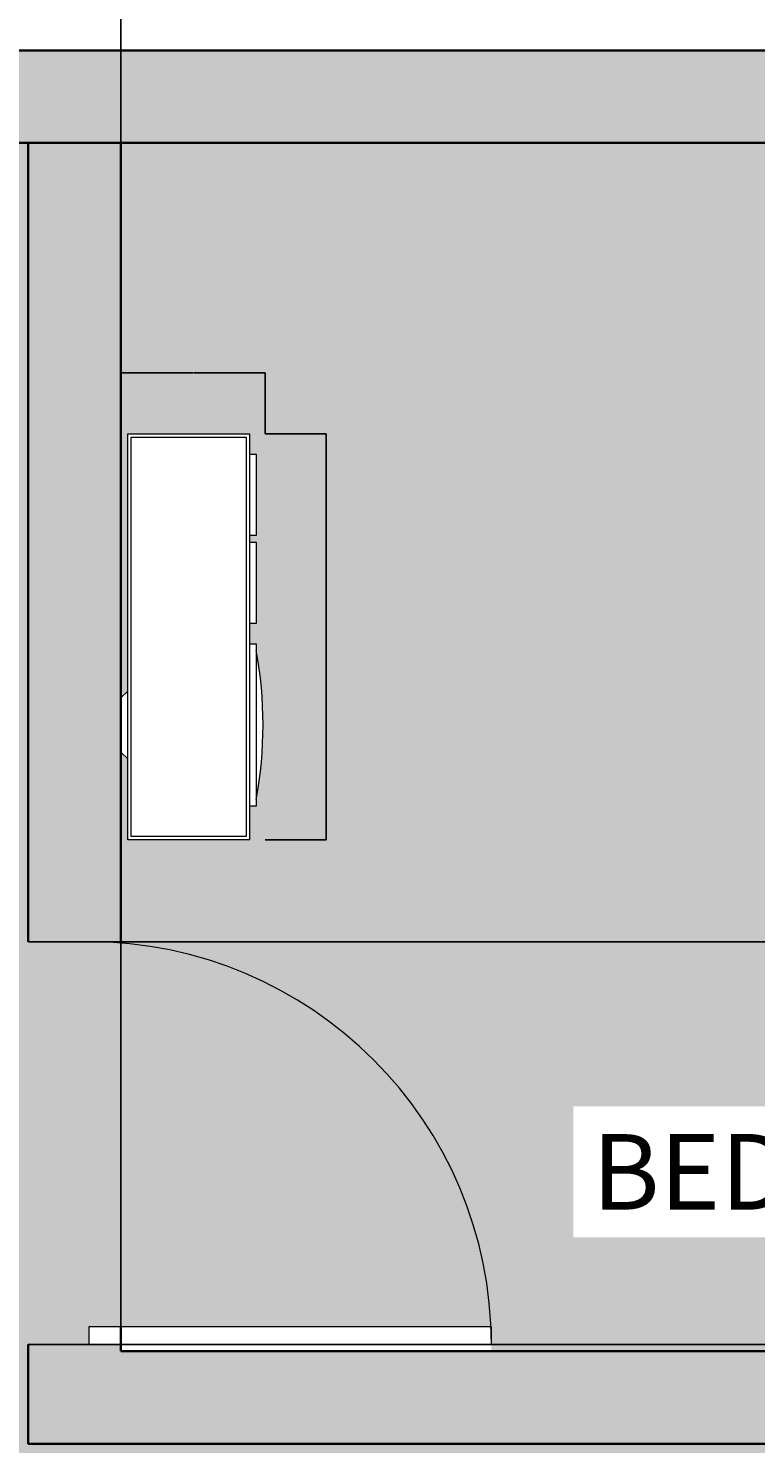
# Model space of a CAD drawing. Units: millimetres. Extents: x -229 to 16545, y -10488 to 4272.
# Tile 26 of 29: x 9556 to 11362, y -1208 to 2307. Entities that reach past the tile are written whole.
import ezdxf

# ---------------------------------------------------------------- set-up
doc = ezdxf.new("R2010")
doc.units = ezdxf.units.MM
for name, color, linetype, lineweight in [('A-ANNO-DIMS', 2, 'Continuous', 18), ('A-AREA-IDEN', 7, 'Continuous', 18), ('A-DOOR', 4, 'Continuous', 18), ('A-FURN', 8, 'Continuous', 18), ('A-WALL', 7, 'Continuous', 35)]:
    doc.layers.add(name, color=color, linetype=linetype, lineweight=lineweight)
doc.layers.add('A-FLOR-PATT', color=254, linetype='Continuous', lineweight=13, true_color=0xfeeab9)
doc.layers.add('A-WALL-PATT', color=18, linetype='Continuous', lineweight=13, true_color=0x000000)
doc.styles.get("Standard").update_dxf_attribs({"font": 'arial.ttf'})
doc.dimstyles.get("Standard").update_dxf_attribs({"dimtxt": 0.18, "dimasz": 0.18, "dimexe": 0.18, "dimexo": 0.0625, "dimgap": 0.09, "dimtad": 0, "dimtih": 1, "dimtoh": 1, "dimdec": 4, "dimzin": 0, "dimdsep": 46, "dimtxsty": 'Standard', "dimcen": 0.09, "dimadec": 0, "dimazin": 0, "dimtfac": 1, "dimtdec": 4, "dimtofl": 0, "dimtmove": 0, "dimatfit": 3, "dimfxl": 1, "dimtolj": 1, "dimtzin": 0, "dimarcsym": 0})

# ---------------------------------------------------------------- blocks, each defined once
blk = doc.blocks.new('Entertainment Center')
for p, q in [((-4, 0), (-5, -1)), ((4, 0), (-4, 0)), ((5, -1), (4, 0)), ((-17, -19), (-17, -1)), ((-17, -1), (43, -1)), ((-16.5, -18.5), (-16.5, -1.5)), ((-16.5, -1.5), (42.5, -1.5)), ((42.5, -1.5), (42.5, -18.5)), ((43, -1), (43, -19)), ((42.5, -18.5), (-16.5, -18.5)), ((43, -19), (-17, -19)), ((-12, -20), (-12, -19)), ((12, -20), (-12, -20)), ((12, -19), (12, -20)), ((15, -20), (15, -19)), ((27, -20), (15, -20)), ((27, -19), (27, -20)), ((28, -20), (28, -19)), ((40, -20), (28, -20)), ((40, -19), (40, -20))]:
    blk.add_line(p, q)
blk.add_arc((0, 40), 61, 259.6111, 280.3889)
blk = doc.blocks.new('*U13')
at = {"transparency": 33554687}
for p, q in [((0, 0), (0, -6)), ((-40, 0), (-40, -6))]:
    blk.add_line(p, q, dxfattribs=at)
blk.add_lwpolyline([(0, 0), (0, 40), (-1.75, 40), (-1.75, 0)], close=True, dxfattribs=at)
blk.add_arc((0, 0), 40, 90, 180, dxfattribs=at)
blk = doc.blocks.new('*D29')
at = {"layer": 'A-ANNO-DIMS', "color": 0, "lineweight": -2, "transparency": 16777216}
for p, q in [((10144.5, 1299.3), (10295.9, 1299.3)), ((10295.8, 1299.1), (10295.8, 795.3)), ((10295.8, 291.1), (10295.8, 794.9)), ((10144.5, 290.9), (10295.9, 290.9))]:
    blk.add_line(p, q, dxfattribs=at)
at = {"layer": 'A-ANNO-DIMS', "color": 0, "transparency": 16777216}
for points in [[(10295.7, 1299.1), (10295.8, 1299.1), (10295.8, 1299.3)], [(10295.7, 291.1), (10295.8, 291.1), (10295.8, 290.9)]]:
    blk.add_solid(points, dxfattribs=at)
at = {"layer": 'Defpoints', "color": 0, "transparency": 16777216}
for p in [(10144.5, 1299.3), (10295.8, 1299.3), (10144.5, 290.9)]:
    blk.add_point(p, dxfattribs=at)
at = {"layer": 'A-ANNO-DIMS', "color": 0, "transparency": 16777216, "insert": (10295.8, 795.1), "char_height": 0.18, "attachment_point": 5}
blk.add_mtext('\\A1;MEDIA UNIT 1008 TYP.', dxfattribs=at)
blk = doc.blocks.new('*D30')
at = {"layer": 'A-ANNO-DIMS', "color": 0, "lineweight": -2, "transparency": 16777216}
for p, q in [((9785.9, 1299.4), (9785.9, 1450.8)), ((9786.1, 1450.6), (9964.6, 1450.6)), ((10144.3, 1450.6), (9965.8, 1450.6)), ((10144.5, 1299.4), (10144.5, 1450.8))]:
    blk.add_line(p, q, dxfattribs=at)
at = {"layer": 'A-ANNO-DIMS', "color": 0, "transparency": 16777216}
for points in [[(9786.1, 1450.6), (9786.1, 1450.6), (9785.9, 1450.6)], [(10144.3, 1450.6), (10144.3, 1450.6), (10144.5, 1450.6)]]:
    blk.add_solid(points, dxfattribs=at)
at = {"layer": 'Defpoints', "color": 0, "transparency": 16777216}
for p in [(9785.9, 1450.6), (9785.9, 1299.3), (10144.5, 1299.3)]:
    blk.add_point(p, dxfattribs=at)
at = {"layer": 'A-ANNO-DIMS', "color": 0, "transparency": 16777216, "insert": (9965.2, 1450.6), "char_height": 0.18, "attachment_point": 5}
blk.add_mtext('\\A1;359 TYP.', dxfattribs=at)
blk = doc.blocks.new('*D45')
at = {"layer": 'A-ANNO-DIMS', "color": 0, "lineweight": -2, "transparency": 16777216}
for p, q in [((2015.9, 2251.8), (2015.9, 4271.7)), ((2016.1, 4271.5), (8015.5, 4271.5)), ((14015.8, 4271.5), (8016.4, 4271.5)), ((14015.9, 2251.8), (14015.9, 4271.7))]:
    blk.add_line(p, q, dxfattribs=at)
at = {"layer": 'A-ANNO-DIMS', "color": 0, "transparency": 16777216}
for points in [[(2016.1, 4271.5), (2016.1, 4271.4), (2015.9, 4271.5)], [(14015.8, 4271.5), (14015.8, 4271.4), (14015.9, 4271.5)]]:
    blk.add_solid(points, dxfattribs=at)
at = {"layer": 'Defpoints', "color": 0, "transparency": 16777216}
for p in [(14015.9, 4271.5), (2015.9, 2251.7), (14015.9, 2251.7)]:
    blk.add_point(p, dxfattribs=at)
at = {"layer": 'A-ANNO-DIMS', "color": 0, "transparency": 16777216, "insert": (8015.9, 4271.5), "char_height": 0.18, "attachment_point": 5}
blk.add_mtext('\\A1;12000', dxfattribs=at)
blk = doc.blocks.new('*D52')
at = {"layer": 'A-ANNO-DIMS', "color": 0, "lineweight": -2, "transparency": 16777216}
for p, q in [((9785.9, -978.2), (9785.9, 4271.7)), ((9786.1, 4271.5), (11785.6, 4271.5)), ((13785.8, 4271.5), (11786.3, 4271.5)), ((13785.9, -978.2), (13785.9, 4271.7))]:
    blk.add_line(p, q, dxfattribs=at)
at = {"layer": 'A-ANNO-DIMS', "color": 0, "transparency": 16777216}
for points in [[(9786.1, 4271.5), (9786.1, 4271.4), (9785.9, 4271.5)], [(13785.8, 4271.5), (13785.8, 4271.4), (13785.9, 4271.5)]]:
    blk.add_solid(points, dxfattribs=at)
at = {"layer": 'Defpoints', "color": 0, "transparency": 16777216}
for p in [(13785.9, 4271.5), (9785.9, -978.3), (13785.9, -978.3)]:
    blk.add_point(p, dxfattribs=at)
at = {"layer": 'A-ANNO-DIMS', "color": 0, "transparency": 16777216, "insert": (11785.9, 4271.5), "char_height": 0.18, "attachment_point": 5}
blk.add_mtext('\\A1;4000', dxfattribs=at)
blk = doc.blocks.new('*D66')
at = {"layer": 'A-ANNO-DIMS', "color": 0, "lineweight": -2, "transparency": 16777216}
for p, q in [((9556, 38.2), (16544.5, 38.2)), ((16544.3, 38), (16544.3, -461.6)), ((16544.3, -961.6), (16544.3, -462)), ((9556, -961.8), (16544.5, -961.8))]:
    blk.add_line(p, q, dxfattribs=at)
at = {"layer": 'A-ANNO-DIMS', "color": 0, "transparency": 16777216}
for points in [[(16544.3, 38), (16544.4, 38), (16544.3, 38.2)], [(16544.3, -961.6), (16544.4, -961.6), (16544.3, -961.8)]]:
    blk.add_solid(points, dxfattribs=at)
at = {"layer": 'Defpoints', "color": 0, "transparency": 16777216}
for p in [(9555.9, 38.2), (9555.9, -961.8), (16544.3, -961.8)]:
    blk.add_point(p, dxfattribs=at)
at = {"layer": 'A-ANNO-DIMS', "color": 0, "transparency": 16777216, "insert": (16544.3, -461.8), "char_height": 0.18, "attachment_point": 5}
blk.add_mtext('\\A1;1000', dxfattribs=at)

msp = doc.modelspace()

# ---------------------------------------------------------------- hatches: boundary and pattern name
at = {"layer": 'A-FLOR-PATT', "transparency": 33554592}
h = msp.add_hatch(color=256, dxfattribs=at)
h.dxf.hatch_style = 1
h.paths.add_polyline_path([(7975.933, -5325.772), (7943.121, -5325.772), (7943.121, -4576.49, 0.40145271), (7225.933, -5325.772, 0.40145271), (6508.746, -4576.49), (6508.746, -5325.772), (6475.933, -5325.772), (6475.933, -5438.272), (5975.933, -5438.272), (5975.933, -7267.724), (5975.933, -7438.272), (6478.619, -7438.272), (6463.448, -7355.919), (6464.88, -7356.837), (6463.849, -7358.097), (6478.619, -7438.272), (6610.327, -7438.272), (6632.656, -7409.564), (6632.525, -7406.967), (6634.208, -7407.569), (6619.273, -7426.77), (6654.466, -7438.272), (7610.517, -7438.272), (7607.41, -7421.409), (7608.842, -7422.327), (7607.812, -7423.587), (7610.517, -7438.272), (7975.933, -7438.272)])
h.paths.add_polyline_path([(13785.933, -1208.272), (9555.933, -1208.272), (9555.933, -961.785), (9705.933, -961.785), (9705.933, -918.035), (10704.976, -918.035, 0.40145271), (9705.933, 38.215), (9555.933, 38.215), (9555.933, 2021.728), (5975.933, 2021.728), (5975.933, 755.492), (5745.933, 755.492), (5745.933, 1427.266), (2918.813, 1427.266), (2918.813, -492.942), (5013.319, -492.942), (5013.319, -978.272), (5745.933, -978.272), (5745.933, -397.513), (5975.933, -397.513), (5975.933, -1208.272), (4560.933, -1208.272), (4560.933, -1265.772), (4448.433, -1265.772), (4448.433, -1298.585), (4445.933, -1298.585), (3699.151, -1298.585, 0.40145271), (4448.433, -2015.772), (4560.933, -2015.772), (4560.933, -2384.177), (5745.933, -2384.177), (5799.402, -2384.177), (5799.402, -4518.272), (5975.933, -4518.272), (5975.933, -5208.272), (6475.933, -5208.272), (6475.933, -4575.772), (6508.746, -4575.772), (6508.746, -4576.49, -0.35647263), (7216.672, -5208.272), (7235.194, -5208.272, -0.35647263), (7943.121, -4576.49), (7943.121, -4575.772), (7975.933, -4575.772), (7975.933, -5208.272), (11176.247, -5208.272), (11159.44, -5191.465), (10520.768, -5191.465), (10520.768, -4888.936), (10571.19, -4888.936), (10571.19, -4872.129), (10772.876, -4872.129), (10772.876, -4888.936), (10789.683, -4888.936), (10789.683, -4872.129), (10991.368, -4872.129), (10991.368, -4888.936), (11041.79, -4888.936), (11041.79, -4872.129), (11058.597, -4872.129, -0.09090909), (11428.354, -4872.129), (11445.162, -4872.129), (11445.162, -4888.936), (11529.197, -4888.936), (11529.197, -5191.465), (11327.512, -5191.465), (11310.704, -5208.272), (13785.933, -5208.272)])
h.paths.add_polyline_path([(11047.216, -1630.944, -1), (11402.816, -1630.944, -1)], flags=16)
h.paths.add_polyline_path([(11148.816, -1630.944), (11225.016, -1554.744), (11301.216, -1630.944), (11225.016, -1707.144)], flags=0)
h.paths.add_polyline_path([(11199.616, -1630.944, -1), (11250.416, -1630.944, -1)], flags=0)
h.paths.add_polyline_path([(11588.751, -2096.259), (11588.751, -1543.254, -0.26666697), (12864.918, -1543.254), (12864.918, -2096.259), (12737.302, -2096.259), (12737.302, -2063.121), (11716.368, -2063.121), (11716.368, -2096.259)], flags=16)
h.paths.add_polyline_path([(12012.696, -2489.42), (12600.997, -2489.42), (12600.997, -3666.022), (12012.696, -3666.022)], flags=16)
h.paths.add_polyline_path([(12176.41, -3599.403), (12174.938, -3609.076), (12173.789, -3618.819), (12173.09, -3628.559), (12172.973, -3638.221), (12173.89, -3652.852), (12175.008, -3657.025), (12172.909, -3643.473), (12173.142, -3624.297), (12175.386, -3605.273)], flags=0)
h.paths.add_polyline_path([(8026.289, -286.944), (7737.703, -287.19), (7734.87, -269.156), (8029.092, -268.905)], flags=16)
h.paths.add_polyline_path([(7733.453, -260.139), (7710.784, -115.865), (7557.191, -115.996), (7556.999, 109.744), (7412.687, 132.166), (7412.433, 429.206), (7556.707, 451.876), (7556.568, 614.769), (7412.256, 637.19), (7412.003, 934.231), (7556.276, 956.9), (7556.084, 1182.639), (7709.677, 1182.77), (7732.099, 1327.082), (8029.14, 1327.335), (8051.808, 1183.062), (8205.401, 1183.192), (8205.594, 957.454), (8349.906, 935.031), (8350.159, 637.99), (8205.885, 615.322), (8206.024, 452.43), (8350.336, 430.006), (8350.59, 132.965), (8206.316, 110.298), (8206.509, -115.442), (8052.916, -115.573), (8030.493, -259.885)], flags=16)
h.paths.add_polyline_path([(12261.416, -3475.554), (12262.632, -3486.776), (12264.032, -3497.007), (12265.554, -3506.365), (12267.136, -3514.968), (12268.719, -3522.935), (12271.304, -3535.59), (12273.606, -3548.078), (12275.271, -3561.064), (12275.93, -3574.938), (12275.325, -3590.3), (12273.425, -3607.964), (12270.795, -3625.658), (12268.066, -3641.063), (12266.318, -3649.679), (12265.456, -3653.626), (12263.984, -3659.846), (12264.032, -3659.566), (12264.342, -3658.241), (12264.807, -3656.37), (12265.456, -3653.626), (12266.318, -3649.679), (12267.409, -3644.302), (12268.668, -3637.664), (12270.019, -3630.037), (12271.384, -3621.695), (12272.69, -3612.908), (12273.857, -3603.948), (12274.81, -3595.088), (12275.47, -3586.601), (12275.782, -3578.689), (12275.757, -3571.292), (12275.423, -3564.275), (12274.816, -3557.512), (12273.964, -3550.872), (12272.896, -3544.224), (12271.645, -3537.439), (12270.24, -3530.385), (12267.543, -3517.181), (12264.612, -3501.247), (12261.849, -3481.059)], flags=0)
h.paths.add_polyline_path([(12332.136, -3408.03), (12333.483, -3416.79), (12335.077, -3424.54), (12336.915, -3431.355), (12338.991, -3437.32), (12341.266, -3442.55), (12343.694, -3447.166), (12346.229, -3451.292), (12348.826, -3455.051), (12351.438, -3458.563), (12357.476, -3466.491), (12363.61, -3476.575), (12368.309, -3489.762), (12369.929, -3503.427), (12369.842, -3516.511), (12368.43, -3530.867), (12365.816, -3545.835), (12362.382, -3559.786), (12360.968, -3564.487), (12363.063, -3557.021), (12364.898, -3549.566), (12366.473, -3542.077), (12367.773, -3534.631), (12368.781, -3527.301), (12369.483, -3520.162), (12369.863, -3513.291), (12369.906, -3506.759), (12369.599, -3500.643), (12368.93, -3494.999), (12367.924, -3489.796), (12366.61, -3484.994), (12365.024, -3480.542), (12363.19, -3476.399), (12361.141, -3472.516), (12358.909, -3468.847), (12356.525, -3465.347), (12354.02, -3461.954), (12351.438, -3458.563), (12345.462, -3450.529), (12339.923, -3439.996), (12335.85, -3428.296), (12332.68, -3412.888)], flags=0)
h.paths.add_polyline_path([(12385.287, -3334.612), (12384.977, -3342.409), (12385.02, -3349.196), (12385.4, -3355.066), (12386.104, -3360.105), (12387.112, -3364.41), (12388.412, -3368.071), (12389.987, -3371.181), (12391.823, -3373.832), (12393.919, -3376.097), (12396.337, -3377.978), (12399.153, -3379.462), (12402.445, -3380.531), (12406.289, -3381.172), (12410.758, -3381.371), (12415.935, -3381.106), (12421.893, -3380.368), (12428.658, -3379.159), (12436.069, -3377.55), (12443.907, -3375.635), (12451.961, -3373.505), (12460.015, -3371.254), (12467.853, -3368.971), (12475.263, -3366.749), (12482.029, -3364.68), (12491.877, -3361.657), (12497.701, -3360.107), (12501.639, -3359.288), (12510.135, -3358.326), (12519.662, -3365.412), (12524.243, -3378.911), (12523.764, -3390.7), (12520.746, -3401.577), (12514.248, -3415.634), (12511.518, -3420.418), (12515.856, -3412.154), (12519.153, -3405.024), (12521.516, -3398.804), (12523.049, -3393.276), (12523.865, -3388.212), (12524.059, -3383.441), (12523.7, -3378.958), (12522.853, -3374.815), (12521.576, -3371.054), (12519.931, -3367.722), (12517.982, -3364.865), (12515.786, -3362.529), (12513.405, -3360.758), (12510.877, -3359.588), (12508.136, -3358.982), (12505.086, -3358.897), (12501.639, -3359.288), (12497.701, -3360.107), (12493.183, -3361.309), (12487.988, -3362.851), (12476.403, -3366.408), (12463.335, -3370.326), (12447.372, -3374.788), (12431.759, -3378.604), (12418.504, -3380.974), (12405.811, -3381.624), (12394.725, -3378.025), (12388.039, -3368.367), (12385.583, -3357.877), (12384.826, -3346.204), (12385.428, -3331.059), (12385.953, -3325.719)], flags=0)
h.paths.add_polyline_path([(7880.016, 1173.969), (7880.373, 1175.495), (7880.433, 1175.851), (7879.484, 1171.818)], flags=0)
h.paths.add_polyline_path([(7802.33, 874.962), (7800.771, 885.032), (7798.932, 893.941), (7796.811, 901.774), (7794.419, 908.63), (7791.798, 914.639), (7789.002, 919.945), (7786.083, 924.686), (7783.093, 929.005), (7780.087, 933.043), (7774.996, 939.717), (7768.406, 949.37), (7762.174, 963.427), (7759.342, 978.002), (7758.629, 991.888), (7759.492, 1007.928), (7761.801, 1025.496), (7765.392, 1044.035), (7766.625, 1049.048), (7764.522, 1039.543), (7762.719, 1030.232), (7761.232, 1021.168), (7760.08, 1012.405), (7759.28, 1003.994), (7758.849, 995.988), (7758.806, 988.44), (7759.167, 981.404), (7759.942, 974.914), (7761.104, 968.936), (7762.617, 963.414), (7764.448, 958.299), (7766.559, 953.535), (7768.918, 949.073), (7771.487, 944.856), (7774.232, 940.835), (7777.115, 936.938), (7782.377, 930.041), (7787.845, 922.139), (7793.348, 911.698), (7798.042, 898.247), (7801.702, 880.527)], flags=0)
h.paths.add_polyline_path([(12519.068, -3228.534), (12519.615, -3236.235), (12520.529, -3242.343), (12521.78, -3247.103), (12523.337, -3250.758), (12525.171, -3253.556), (12527.248, -3255.709), (12529.522, -3257.296), (12531.95, -3258.361), (12534.486, -3258.949), (12537.082, -3259.11), (12539.694, -3258.888), (12542.277, -3258.329), (12544.781, -3257.478), (12547.173, -3256.388), (12549.46, -3255.129), (12550.455, -3254.517), (12555.825, -3251.109), (12557.835, -3249.942), (12565.181, -3246.404), (12574.565, -3253.032), (12576.931, -3265.022), (12576.627, -3277.425), (12575.416, -3290.819), (12574.851, -3295.392), (12575.708, -3287.593), (12576.322, -3280.806), (12576.688, -3274.939), (12576.812, -3269.899), (12576.688, -3265.593), (12576.322, -3261.932), (12575.708, -3258.822), (12574.851, -3256.172), (12573.753, -3253.905), (12572.439, -3252.005), (12570.943, -3250.474), (12569.293, -3249.309), (12567.523, -3248.513), (12565.658, -3248.083), (12563.732, -3248.022), (12561.777, -3248.328), (12559.814, -3248.989), (12557.835, -3249.942), (12555.825, -3251.109), (12553.77, -3252.413), (12551.652, -3253.78), (12549.46, -3255.129), (12543.167, -3258.594), (12532.661, -3259.485), (12524.685, -3253.923), (12520.949, -3245.152), (12519.138, -3233.042)], flags=0)
h.paths.add_polyline_path([(7741.293, 790.501), (7741.641, 799.467), (7741.584, 807.269), (7741.141, 814.015), (7740.329, 819.809), (7739.165, 824.757), (7737.667, 828.966), (7735.853, 832.541), (7733.74, 835.586), (7731.348, 838.188), (7728.71, 840.348), (7725.861, 842.052), (7722.836, 843.28), (7719.671, 844.015), (7716.4, 844.237), (7713.06, 843.932), (7709.684, 843.081), (7706.304, 841.686), (7702.923, 839.834), (7699.543, 837.629), (7696.164, 835.178), (7692.784, 832.585), (7684.718, 826.315), (7675.609, 820.63), (7664.001, 817.274), (7654.105, 821.884), (7647.171, 832.02), (7644.191, 846.522), (7646.321, 860.288), (7647.49, 864.223), (7645.946, 857.865), (7645.046, 852.044), (7644.827, 846.557), (7645.243, 841.404), (7646.221, 836.642), (7647.693, 832.318), (7649.587, 828.489), (7651.832, 825.206), (7654.359, 822.523), (7657.097, 820.49), (7659.984, 819.145), (7662.993, 818.452), (7666.108, 818.357), (7669.311, 818.809), (7672.583, 819.755), (7675.908, 821.139), (7679.268, 822.913), (7682.645, 825.021), (7686.025, 827.401), (7689.404, 829.958), (7692.784, 832.585), (7700.505, 838.509), (7709.871, 843.64), (7721.436, 844.698), (7733.277, 837.617), (7739.571, 825.214), (7741.557, 811.049), (7741.669, 795.575)], flags=0)
h.paths.add_polyline_path([(8377.641, 137.216), (8359.607, 134.382), (8359.356, 428.605), (8377.395, 425.802)], flags=16)
h.paths.add_polyline_path([(7650.715, 668.465), (7650.08, 677.319), (7649.023, 684.34), (7647.579, 689.811), (7645.785, 694.012), (7643.675, 697.228), (7641.286, 699.7), (7638.669, 701.521), (7635.876, 702.744), (7632.96, 703.419), (7629.974, 703.601), (7626.971, 703.344), (7624.004, 702.697), (7621.125, 701.717), (7618.375, 700.462), (7615.749, 699.013), (7614.561, 698.279), (7608.435, 694.382), (7606.125, 693.04), (7598.981, 689.594), (7589.669, 693.773), (7585.26, 702.856), (7584.221, 713.11), (7584.49, 724.584), (7585.863, 739.937), (7586.518, 745.277), (7585.539, 736.31), (7584.841, 728.507), (7584.424, 721.761), (7584.288, 715.966), (7584.433, 711.016), (7584.86, 706.807), (7585.567, 703.231), (7586.556, 700.186), (7587.821, 697.58), (7589.332, 695.397), (7591.053, 693.637), (7592.951, 692.3), (7594.989, 691.385), (7597.132, 690.895), (7599.346, 690.826), (7601.594, 691.18), (7603.851, 691.943), (7606.125, 693.04), (7608.435, 694.382), (7610.797, 695.885), (7613.229, 697.458), (7620.475, 701.929), (7632.001, 704.44), (7643.476, 699.417), (7648.536, 687.571), (7650.63, 673.661)], flags=0)
h.paths.add_polyline_path([(7385.628, 136.37), (7385.382, 424.956), (7403.416, 427.789), (7403.667, 133.567)], flags=16)
h.paths.add_polyline_path([(12993.884, -2257.186), (12959.588, -2257.186), (12959.588, -2125.099), (13531.966, -2125.099, -0.19047621), (13531.966, -3974.321), (12959.588, -3974.321), (12959.588, -3842.233), (12993.884, -3842.233)], flags=16)
h.paths.add_polyline_path([(13413.486, -3313.884), (13413.486, -2785.535), (13562.885, -2785.535, -0.04962821), (13562.885, -3313.884)], flags=0)
h.paths.add_polyline_path([(8377.21, 642.241), (8359.176, 639.407), (8358.925, 933.629), (8376.964, 930.826)], flags=16)
h.paths.add_polyline_path([(13086.058, -1864.83), (13086.058, -1449.84), (13501.048, -1449.84), (13501.048, -1864.83)], flags=16)
h.paths.add_polyline_path([(13305.814, -1862.197), (13302.103, -1859.624), (13298.088, -1857.068), (13293.799, -1854.536), (13289.262, -1852.031), (13284.504, -1849.559), (13279.554, -1847.125), (13274.439, -1844.735), (13269.17, -1842.389), (13263.701, -1840.081), (13257.97, -1837.797), (13251.914, -1835.525), (13245.472, -1833.252), (13238.582, -1830.968), (13231.18, -1828.66), (13223.206, -1826.315), (13209.182, -1822.458), (13204.584, -1821.48), (13217.962, -1824.773), (13235.072, -1829.804), (13248.777, -1834.349), (13260.829, -1838.869), (13274.479, -1844.63), (13289.675, -1852.101), (13302.553, -1859.704)], flags=0)
h.paths.add_polyline_path([(13428.104, -1820.994), (13419.007, -1818.141), (13409.95, -1815.4), (13400.766, -1812.747), (13391.271, -1810.151), (13376.087, -1806.251), (13370.618, -1805.019), (13386.304, -1808.794), (13405.087, -1813.928), (13423.014, -1819.354)], flags=0)
h.paths.add_polyline_path([(7385.197, 641.395), (7384.951, 929.98), (7402.986, 932.814), (7403.236, 638.592)], flags=16)
h.paths.add_polyline_path([(13262.537, -1725.526), (13253.246, -1724.74), (13244.516, -1724.117), (13235.94, -1723.625), (13223.267, -1723.062), (13217.598, -1722.912), (13231.966, -1723.397), (13248.733, -1724.359), (13266.899, -1725.895), (13272.802, -1726.502)], flags=0)
h.paths.add_polyline_path([(13191.893, -1641.137), (13208.675, -1640.506), (13214.057, -1640.258), (13197.763, -1640.936)], flags=0)
h.paths.add_polyline_path([(13097.524, -1608.457), (13114.284, -1609.031), (13120.126, -1609.105), (13103.045, -1608.71)], flags=0)
h.paths.add_polyline_path([(13465.328, -1521.577), (13473.906, -1517.015), (13481.761, -1511.636), (13492.562, -1502.076), (13495.327, -1497.933), (13485.818, -1508.858), (13470.208, -1519.547)], flags=0)
h.paths.add_polyline_path([(13175.015, -1500.891), (13184.046, -1501.807), (13192.721, -1502.52), (13201.114, -1503.034), (13209.273, -1503.351), (13217.244, -1503.476), (13225.078, -1503.41), (13232.821, -1503.16), (13240.524, -1502.728), (13248.233, -1502.117), (13255.993, -1501.322), (13263.825, -1500.293), (13271.746, -1498.974), (13279.775, -1497.305), (13287.928, -1495.229), (13296.222, -1492.688), (13304.675, -1489.622), (13313.304, -1485.975), (13322.089, -1481.727), (13330.859, -1477.028), (13339.408, -1472.063), (13347.526, -1467.02), (13355.006, -1462.087), (13364.86, -1455.202), (13367.224, -1453.299), (13358.544, -1459.754), (13343.348, -1469.775), (13326.143, -1479.767), (13309.023, -1488.045), (13292.249, -1494.129), (13276.009, -1498.264), (13260.299, -1500.88), (13244.401, -1502.51), (13228.945, -1503.378), (13213.316, -1503.508), (13197.047, -1502.876), (13180.088, -1501.481)], flags=0)
h.paths.add_polyline_path([(7733.501, 1336.101), (7736.303, 1354.14), (8024.889, 1354.386), (8027.723, 1336.352)], flags=16)
h = msp.add_hatch(color=256, dxfattribs=at)
h.dxf.hatch_style = 1
h.paths.add_polyline_path([(13785.933, 2021.728), (9555.933, 2021.728), (9555.933, 38.215), (9705.933, 38.215, -0.40145271), (10704.976, -918.035), (10705.933, -918.035), (10705.933, -978.272), (13785.933, -978.272)])
h.paths.add_polyline_path([(12170.451, 1206.716), (13722.905, 1206.716), (13722.905, 42.377), (12170.451, 42.377)], flags=16)
h.paths.add_polyline_path([(10122.076, 374.936), (10105.269, 374.936), (10105.269, 290.901), (9802.74, 290.901), (9802.74, 492.586), (9785.933, 509.394), (9785.933, 643.851), (9802.74, 660.658), (9802.74, 1299.33), (10105.269, 1299.33), (10105.269, 1248.908), (10122.076, 1248.908), (10122.076, 1047.222), (10105.269, 1047.222), (10105.269, 1030.415), (10122.076, 1030.415), (10122.076, 828.729), (10105.269, 828.729), (10105.269, 778.308), (10122.076, 778.308), (10122.076, 761.501, -0.09090909), (10122.076, 391.743)], flags=16)
h.paths.add_polyline_path([(10096.865, 299.304), (9811.144, 299.304), (9811.144, 1290.926), (10096.865, 1290.926)], flags=0)
h.paths.add_polyline_path([(13148.497, 337.342), (13443.463, 337.342), (13443.463, 1051.471), (13699.618, 1051.471), (13699.618, 647.833), (13443.463, 647.833), (13443.463, 601.26), (13699.618, 601.26), (13699.618, 197.622), (13404.652, 197.622), (13404.652, 298.531), (13148.497, 42.377)], flags=0)
h.paths.add_polyline_path([(13445.876, -25.215), (13737.804, -25.215), (13737.804, -349.58), (13445.876, -349.58)], flags=16)
h.paths.add_polyline_path([(13462.094, -41.433), (13559.404, -41.433), (13559.404, -122.524), (13535.076, -122.524), (13535.076, -260.379), (13551.295, -260.379), (13551.295, -333.361), (13470.203, -333.361), (13470.203, -260.379), (13486.422, -260.379), (13486.422, -122.524), (13462.094, -122.524)], flags=0)
h.paths.add_polyline_path([(13575.622, -73.869), (13721.586, -73.869), (13721.586, -138.742), (13575.622, -138.742)], flags=0)
h.paths.add_polyline_path([(13616.168, -219.834), (13681.04, -219.834), (13681.04, -317.143), (13616.168, -317.143)], flags=0)
h.paths.add_polyline_path([(13371.868, 1425.214, -1), (13727.468, 1425.214, -1)], flags=16)
h.paths.add_polyline_path([(13473.468, 1425.214), (13549.668, 1501.414), (13625.868, 1425.214), (13549.668, 1349.014)], flags=0)
h.paths.add_polyline_path([(13524.268, 1425.214, -1), (13575.068, 1425.214, -1)], flags=0)
at = {"layer": 'A-WALL-PATT'}
h = msp.add_hatch(color=256, dxfattribs=at)
h.dxf.hatch_style = 1
h.paths.add_polyline_path([(7294.425, 2163.983), (7294.425, 2251.728), (4412.722, 2251.728), (4412.722, 2166.741), (4412.722, 2122.457), (4412.722, 2021.728), (7294.425, 2021.728), (7294.425, 2119.698)])
h.paths.add_polyline_path([(11407.51, 2166.741), (11407.51, 2251.728), (8296.763, 2251.728), (8296.763, 2163.983), (8296.763, 2119.698), (8296.763, 2021.728), (11407.51, 2021.728), (11407.51, 2122.457)])
h.paths.add_polyline_path([(9785.933, 2021.728), (9555.933, 2021.728), (9555.933, 38.215), (9705.933, 38.215, -0.02002407), (9785.933, 35.01)])
h.paths.add_polyline_path([(14015.933, 2251.728), (12488.002, 2251.728), (12488.002, 2166.742), (12488.002, 2122.738), (12488.002, 2021.728), (13785.933, 2021.728), (13785.933, -2305.465), (13883.903, -2305.465), (13928.188, -2305.465), (14015.933, -2305.465)])
h.paths.add_polyline_path([(13785.933, -978.272), (9785.933, -978.272), (9785.933, -961.785), (9705.933, -961.785), (9555.933, -961.785), (9555.933, -1208.272), (13785.933, -1208.272)])
h.paths.add_polyline_path([(5975.933, 2021.728), (5745.933, 2021.728), (5745.933, 755.492), (5975.933, 755.492)])
h.paths.add_polyline_path([(2245.933, 2021.728), (3420.865, 2021.728), (3420.865, 2122.457), (3420.865, 2167.104), (3420.865, 2251.728), (2015.933, 2251.728), (2015.933, -3326.811), (2100.943, -3326.811), (2155.199, -3326.811), (2245.933, -3326.811)])
h.paths.add_polyline_path([(5975.933, -397.513), (5745.933, -397.513), (5745.933, -978.272), (2245.933, -978.272), (2245.933, -1208.272), (5975.933, -1208.272)])
h.paths.add_polyline_path([(12015.17, -5208.272), (7975.933, -5208.272), (7975.933, -5325.772), (7975.933, -5438.272), (7975.933, -5596.884), (8205.933, -5596.884), (8205.933, -5438.272), (12015.17, -5438.272), (12015.17, -5337.543), (12015.17, -5293.259)])
h.paths.add_polyline_path([(5975.933, -4518.272), (4567.83, -4518.272), (4567.83, -4603.259), (4567.83, -4647.543), (4567.83, -4748.272), (5745.933, -4748.272), (5745.933, -5438.272), (5975.933, -5438.272), (6475.933, -5438.272), (6475.933, -5325.772), (6475.933, -5208.272), (5975.933, -5208.272)])
h.paths.add_polyline_path([(3765.491, -4518.272), (2245.933, -4518.272), (2245.933, -4748.272), (3765.491, -4748.272), (3765.491, -4647.543), (3765.491, -4603.259)])

# ---------------------------------------------------------------- linework, layer by layer
at = {"layer": 'A-WALL'}
for p, q in [((2015.933, 2251.728), (14015.933, 2251.728)), ((2245.933, 2021.728), (13785.933, 2021.728)), ((9555.933, 2021.728), (9555.933, 38.215)), ((9785.933, 2021.728), (9785.933, 35.01)), ((9785.933, -918.035), (9785.933, -978.272)), ((9555.933, -961.785), (9555.933, -1208.272)), ((9785.933, -978.272), (13785.933, -978.272)), ((9555.933, -1208.272), (13785.933, -1208.272))]:
    msp.add_line(p, q, dxfattribs=at)

# ---------------------------------------------------------------- block references
at = {"layer": 'A-DOOR', "xscale": 25, "yscale": 25, "zscale": 25, "rotation": 270}
msp.add_blockref('*U13', (9705.933, -961.785), dxfattribs=at)
at = {"layer": 'A-FURN', "xscale": 16.80715229332562, "yscale": 16.80715229332562, "zscale": 16.80715229332562, "rotation": 89.99999999999996}
msp.add_blockref('Entertainment Center', (9785.933, 576.622), dxfattribs=at)

# ---------------------------------------------------------------- dimensions: what is measured, and where the dimension line sits
at = {"layer": 'A-ANNO-DIMS'}
dim = msp.add_linear_dim(base=(14015.933, 4271.479), p1=(2015.933, 2251.728), p2=(14015.933, 2251.728), dimstyle='Standard', override={"dimdec": 0, "dimlfac": 1, "dimrnd": 0, "dimzin": 0, "dimdsep": 46, "dimlunit": 2}, dxfattribs=at)
dim.commit()
dim.dimension.update_dxf_attribs({"geometry": '*D45', "text_midpoint": (8015.933, 4271.479)})
for base, p1, p2, angle, text, picture, middle in [((9785.933, 1450.594), (10144.486, 1299.33), (9785.933, 1299.33), 180, '<> TYP.', '*D30', (9965.209, 1450.594)), ((10295.75, 1299.33), (10144.486, 290.901), (10144.486, 1299.33), 90, 'MEDIA UNIT <> TYP.', '*D29', (10295.75, 795.115))]:
    dim = msp.add_linear_dim(base=base, p1=p1, p2=p2, angle=angle, text=text, dimstyle='Standard', override={"dimdec": 0, "dimlfac": 1, "dimrnd": 0, "dimzin": 0, "dimdsep": 46, "dimlunit": 2}, dxfattribs=at)
    dim.commit()
    dim.dimension.update_dxf_attribs({"geometry": picture, "text_midpoint": middle})

# ---------------------------------------------------------------- next in the draw order: wipeouts: each hides what was drawn before it
msp.add_wipeout([(10909.115, -695.959), (12356.471, -695.959), (12356.471, -370.307), (10909.115, -370.307)]).dxf.layer = 'A-AREA-IDEN'

# ---------------------------------------------------------------- next in the draw order: texts
at = {"layer": 'A-AREA-IDEN'}
msp.add_text('BEDROOM', height=187.719, dxfattribs=at).set_placement((10955.609, -627.057))

# ---------------------------------------------------------------- next in the draw order: dimensions: what is measured, and where the dimension line sits
at = {"layer": 'A-ANNO-DIMS'}
dim = msp.add_linear_dim(base=(13785.933, 4271.479), p1=(9785.933, -978.272), p2=(13785.933, -978.272), dimstyle='Standard', override={"dimdec": 0, "dimlfac": 1, "dimrnd": 0, "dimzin": 0, "dimdsep": 46, "dimlunit": 2}, dxfattribs=at)
dim.commit()
dim.dimension.update_dxf_attribs({"geometry": '*D52', "text_midpoint": (11785.933, 4271.479)})
dim = msp.add_linear_dim(base=(16544.342, -961.785), p1=(9555.933, 38.215), p2=(9555.933, -961.785), angle=90, dimstyle='Standard', override={"dimdec": 0, "dimlfac": 1, "dimrnd": 0, "dimzin": 0, "dimdsep": 46, "dimlunit": 2}, dxfattribs=at)
dim.commit()
dim.dimension.update_dxf_attribs({"geometry": '*D66', "text_midpoint": (16544.342, -461.785)})

doc.saveas('drawing.dxf')
